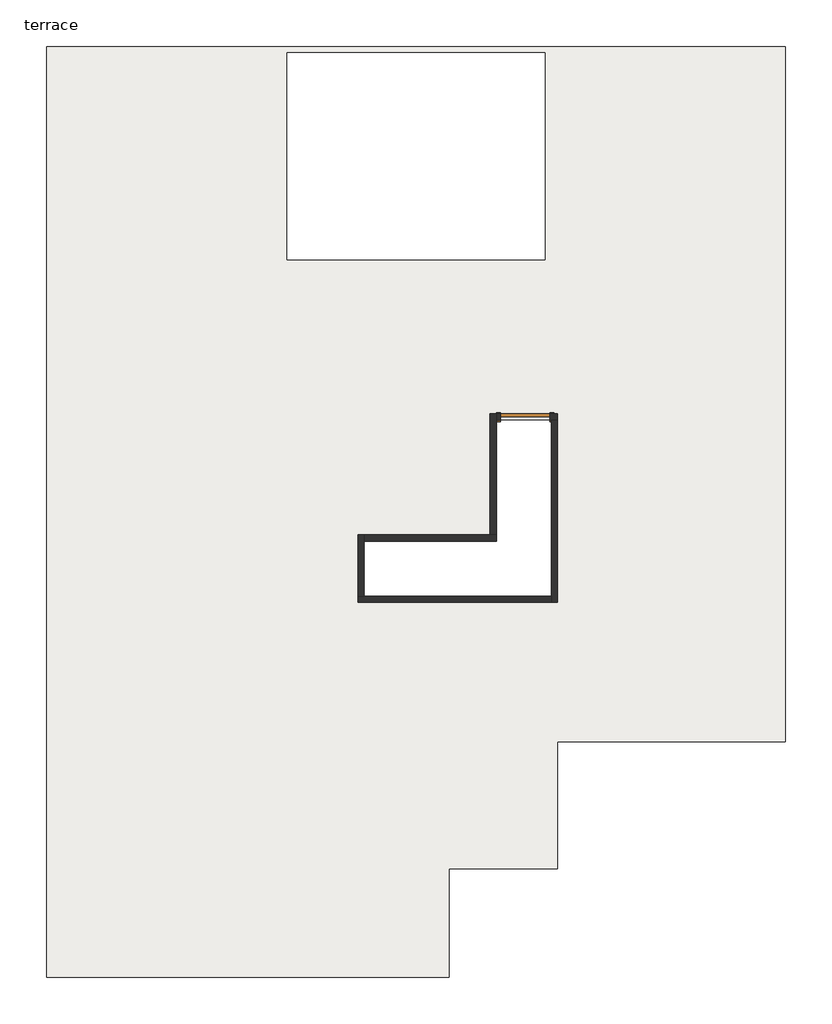
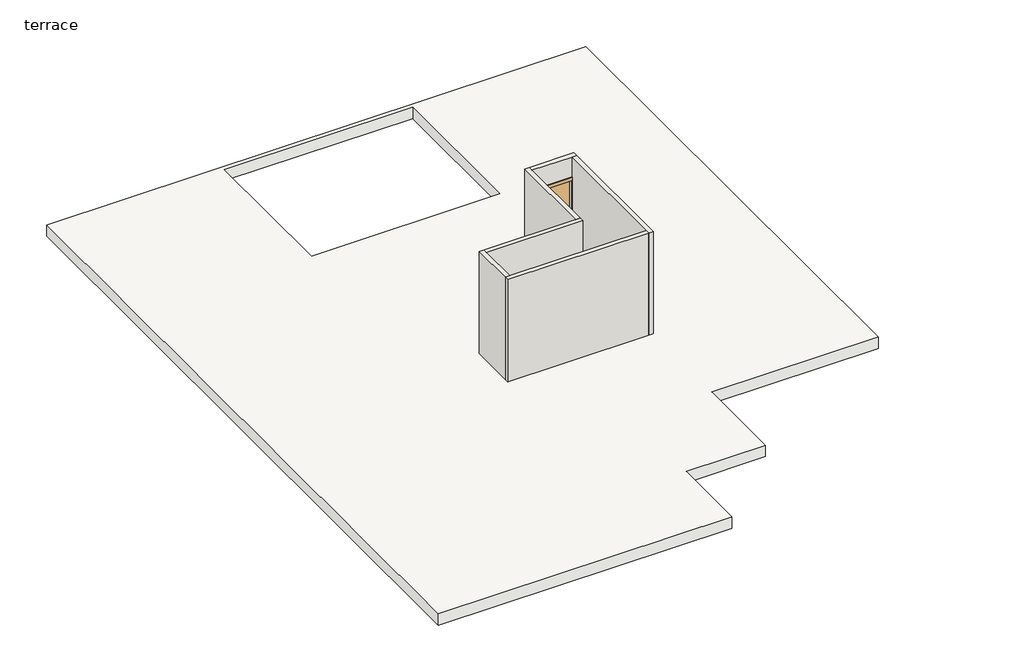
# One storey, incomplete: 6 walls, 1 door, 1 slab.
"""IFC4 building model written with IfcOpenShell, lengths in millimetres."""

from ifc_helpers import new_model, si_unit, frame, origin, place, context, project, spatial, polyline, outline, extrude, faceted_brep, transform, mapped, element, save
from components import door_e5f9f3c4

model = new_model("IFC4")

# Units and contexts
model_context = context("Model", 3, world=origin())
ifc_project = project(units=[si_unit("LENGTHUNIT", "METRE", prefix="MILLI")], contexts=[model_context])

# Site, building, storey
site = spatial("IfcSite", under=ifc_project)
building = spatial("IfcBuilding", under=site)
storey = spatial("IfcBuildingStorey", under=building, Name="terrace", Elevation=3810.0)

# Door
placement = place(None, origin())
door_shape = door_e5f9f3c4(model_context)
element("IfcDoor", 1, ObjectType="Single-Flush : 36\" x 84\"", at=placement, inside=storey, context=model_context, shape_type="MappedRepresentation", body=[
    mapped(door_shape, transform((9562.7120165, 10186.1654956, 3810.0), x_axis=(1.0, 0.0, 0.0), y_axis=(0.0, 1.0, 0.0), z_axis=(0.0, 0.0, 1.0))),
])

# Slab
element("IfcSlab", 2, ObjectType="Generic - 12\"", at=placement, inside=storey, context=model_context, shape_type="SweptSolid", body=[
    extrude(outline(polyline([(14374.3923267, 17035.8496924), (14374.3923267, 4183.4496924), (10157.9923267, 4183.4496924), (10157.9923267, 1833.9496924), (8151.3923267, 1833.9496924), (8151.3923267, -172.6503076), (709.1923267, -172.6503076), (709.1923267, 17035.8496924), (14374.3923267, 17035.8496924)]), holes=[polyline([(5154.1923267, 13098.8496924), (9929.3923267, 13098.8496924), (9929.3923267, 16921.5496924), (5154.1923267, 16921.5496924), (5154.1923267, 13098.8496924)]), polyline([(6584.2175025, 6877.8147181), (10043.6923267, 6877.8147181), (10043.6923267, 10129.0147181), (9027.6923267, 10129.0147181), (9027.6923267, 7893.8147181), (6584.2175025, 7893.8147181), (6584.2175025, 6877.8147181)])]), frame((0.0, 0.0, 3505.2), z_axis=(0.0, 0.0, 1.0), x_axis=(1.0, 0.0, 0.0)), (0.0, 0.0, 1.0), 304.8),
])

# Walls
element("IfcWall", 3, at=placement, inside=storey, context=model_context, shape_type="Brep", body=[
    faceted_brep([(6584.2214491, 7893.8154956, 3810.0), (9027.7808241, 7893.8154956, 3810.0), (9027.7808241, 7893.8154956, 6553.2), (6584.2214491, 7893.8154956, 6553.2), (6584.2214491, 8008.1154956, 3810.0), (6584.2214491, 8008.1154956, 6553.2), (8913.4808241, 8008.1154956, 6553.2), (9027.7808241, 8008.1154956, 6553.2), (9027.7808241, 8008.1154956, 3810.0), (8913.4808241, 8008.1154956, 3810.0)], [[[0, 1, 2, 3]], [[4, 5, 6, 7, 8, 9]], [[1, 0, 4, 9, 8]], [[3, 2, 7, 6, 5]], [[2, 1, 8, 7]], [[0, 3, 5, 4]]]),
])
element("IfcWall", 4, at=placement, inside=storey, context=model_context, shape_type="Brep", body=[
    faceted_brep([(9027.7808241, 8008.1154956, 3810.0), (9027.7808241, 10129.0154956, 3810.0), (9027.7808241, 10243.3154956, 3810.0), (9027.7808241, 10243.3154956, 6553.2), (9027.7808241, 10129.0154956, 6553.2), (9027.7808241, 8008.1154956, 6553.2), (8913.4808241, 8008.1154956, 3810.0), (8913.4808241, 8008.1154956, 6553.2), (8913.4808241, 10243.3154956, 6553.2), (8913.4808241, 10243.3154956, 3810.0)], [[[0, 1, 2, 3, 4, 5]], [[6, 7, 8, 9]], [[2, 1, 0, 6, 9]], [[5, 4, 3, 8, 7]], [[0, 5, 7, 6]], [[3, 2, 9, 8]]]),
])
element("IfcWall", 5, at=placement, inside=storey, context=model_context, shape_type="Brep", body=[
    faceted_brep([(10019.9120165, 10129.0154956, 5943.6), (10019.9120165, 10129.0154956, 3810.0), (10044.1776991, 10129.0154956, 3810.0), (10158.4776991, 10129.0154956, 3810.0), (10158.4776991, 10129.0154956, 6553.2), (10044.1776991, 10129.0154956, 6553.2), (9027.7808241, 10129.0154956, 6553.2), (9027.7808241, 10129.0154956, 3810.0), (9105.5120165, 10129.0154956, 3810.0), (9105.5120165, 10129.0154956, 5943.6), (10158.4776991, 10243.3154956, 3810.0), (10019.9120165, 10243.3154956, 3810.0), (10019.9120165, 10243.3154956, 5943.6), (9105.5120165, 10243.3154956, 5943.6), (9105.5120165, 10243.3154956, 3810.0), (9027.7808241, 10243.3154956, 3810.0), (9027.7808241, 10243.3154956, 6553.2), (10158.4776991, 10243.3154956, 6553.2)], [[[0, 1, 2, 3, 4, 5, 6, 7, 8, 9]], [[10, 11, 12, 13, 14, 15, 16, 17]], [[8, 7, 15, 14]], [[3, 2, 1, 11, 10]], [[6, 5, 4, 17, 16]], [[7, 6, 16, 15]], [[4, 3, 10, 17]], [[12, 11, 1, 0]], [[13, 12, 0, 9]], [[14, 13, 9, 8]]]),
])
element("IfcWall", 6, at=placement, inside=storey, context=model_context, shape_type="Brep", body=[
    faceted_brep([(10044.1776991, 10129.0154956, 3810.0), (10044.1776991, 6877.8154956, 3810.0), (10044.1776991, 6763.5154956, 3810.0), (10044.1776991, 6763.5154956, 6553.2), (10044.1776991, 6877.8154956, 6553.2), (10044.1776991, 10129.0154956, 6553.2), (10158.4776991, 10129.0154956, 3810.0), (10158.4776991, 10129.0154956, 6553.2), (10158.4776991, 6763.5154956, 6553.2), (10158.4776991, 6763.5154956, 3810.0)], [[[0, 1, 2, 3, 4, 5]], [[6, 7, 8, 9]], [[2, 1, 0, 6, 9]], [[5, 4, 3, 8, 7]], [[0, 5, 7, 6]], [[3, 2, 9, 8]]]),
])
element("IfcWall", 7, at=placement, inside=storey, context=model_context, shape_type="Brep", body=[
    faceted_brep([(10044.1776991, 6877.8154956, 3810.0), (6584.2214491, 6877.8154956, 3810.0), (6469.9214491, 6877.8154956, 3810.0), (6469.9214491, 6877.8154956, 6553.2), (6584.2214491, 6877.8154956, 6553.2), (10044.1776991, 6877.8154956, 6553.2), (10044.1776991, 6763.5154956, 3810.0), (10044.1776991, 6763.5154956, 6553.2), (6469.9214491, 6763.5154956, 6553.2), (6469.9214491, 6763.5154956, 3810.0)], [[[0, 1, 2, 3, 4, 5]], [[6, 7, 8, 9]], [[2, 1, 0, 6, 9]], [[5, 4, 3, 8, 7]], [[0, 5, 7, 6]], [[3, 2, 9, 8]]]),
])
element("IfcWall", 8, at=placement, inside=storey, context=model_context, shape_type="Brep", body=[
    faceted_brep([(6584.2214491, 6877.8154956, 3810.0), (6584.2214491, 7893.8154956, 3810.0), (6584.2214491, 8008.1154956, 3810.0), (6584.2214491, 8008.1154956, 6553.2), (6584.2214491, 7893.8154956, 6553.2), (6584.2214491, 6877.8154956, 6553.2), (6469.9214491, 6877.8154956, 3810.0), (6469.9214491, 6877.8154956, 6553.2), (6469.9214491, 8008.1154956, 6553.2), (6469.9214491, 8008.1154956, 3810.0)], [[[0, 1, 2, 3, 4, 5]], [[6, 7, 8, 9]], [[2, 1, 0, 6, 9]], [[5, 4, 3, 8, 7]], [[0, 5, 7, 6]], [[3, 2, 9, 8]]]),
])

save(model, "model.ifc")

# Revit data of these elements
# Type "Single-Flush : 36\" x 84\""
#   Type Mark = "1"
#   Construction Type Id = "MDOOR"
#   Assembly Code = "C1020"
#   Analytic Construction = "Metal"
#   Thickness = 0' - 2"
#   Heat Transfer Coefficient (U) = 0.651978 BTU/(h·ft²·°F)
#   Height = 7' - 0"
#   Trim Projection Ext = 0' - 1"
#   Trim Projection Int = 0' - 1"
#   Trim Width = 0' - 3"
#   Width = 3' - 0"
#   Define Thermal Properties by = 1
#   Define Thermal Properties by = 1
#   Door Material = Door - Panel
#   Frame Material = Door - Frame
#   Visual Light Transmittance = 0
#   Solar Heat Gain Coefficient = 0
#   Function = (empty or 0)
#   Wall Closure = (empty or 0)
# Type "Generic - 12\""
#   Assembly Code = "B1010"
#   Function = 0
#   Layers, outside or top first: 1' - 0" no material (function 1)
# Type
#   Assembly Code = "B2010"
#   Layers, outside or top first: 0' - 4 1/2" no material (function 1)
# Element 1 (IfcDoor, "Single-Flush : 36\" x 84\"")
#   Phase Created = New Construction
#   Materials on its faces: "Door - Frame", "Door - Panel"
# Element 2 (IfcSlab, "Generic - 12\"")
#   Height Offset From Level = 0' - 0"
#   Phase Created = New Construction
#   Materials on its faces: "Default Floor"
# Elements 3, 4, 5, 6, 7, 8 (IfcWall)
#   Top Offset = 0' - 0"
#   Base Offset = 0' - 0"
#   wall height = 9' - 0"
#   Phase Created = New Construction
#   Base Constraint = terrace
#   Top Constraint = stair head room
#   Materials on its faces: "Default Wall"
# Materials
#   "Door - Panel": class "Wood", colour RGB 210 159 95, transparency 0, Cost = 0
#   "Door - Frame": colour RGB 118 70 51, transparency 0, Cost = 0
#   "Default Floor": colour RGB 128 128 128, transparency 0, Cost = 0
#   "Default Wall": colour RGB 128 128 128, transparency 0, Cost = 0
